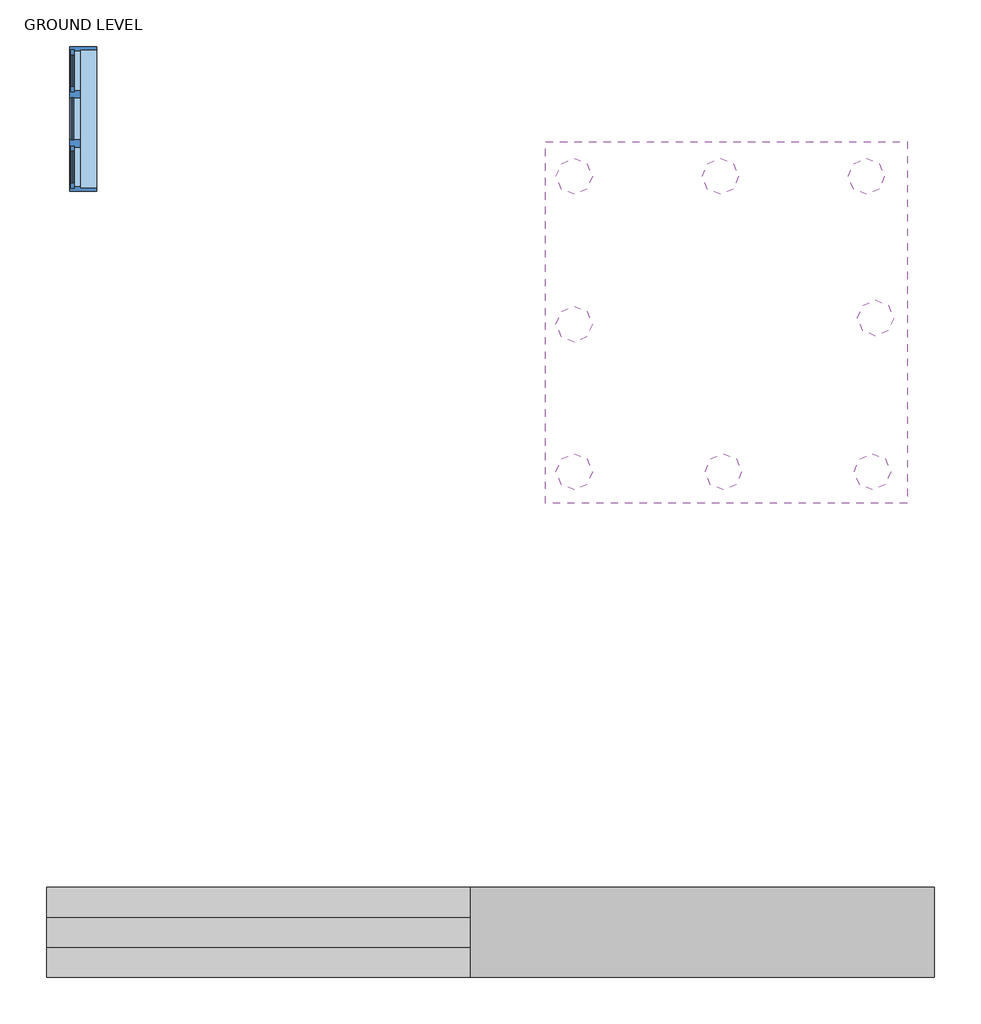
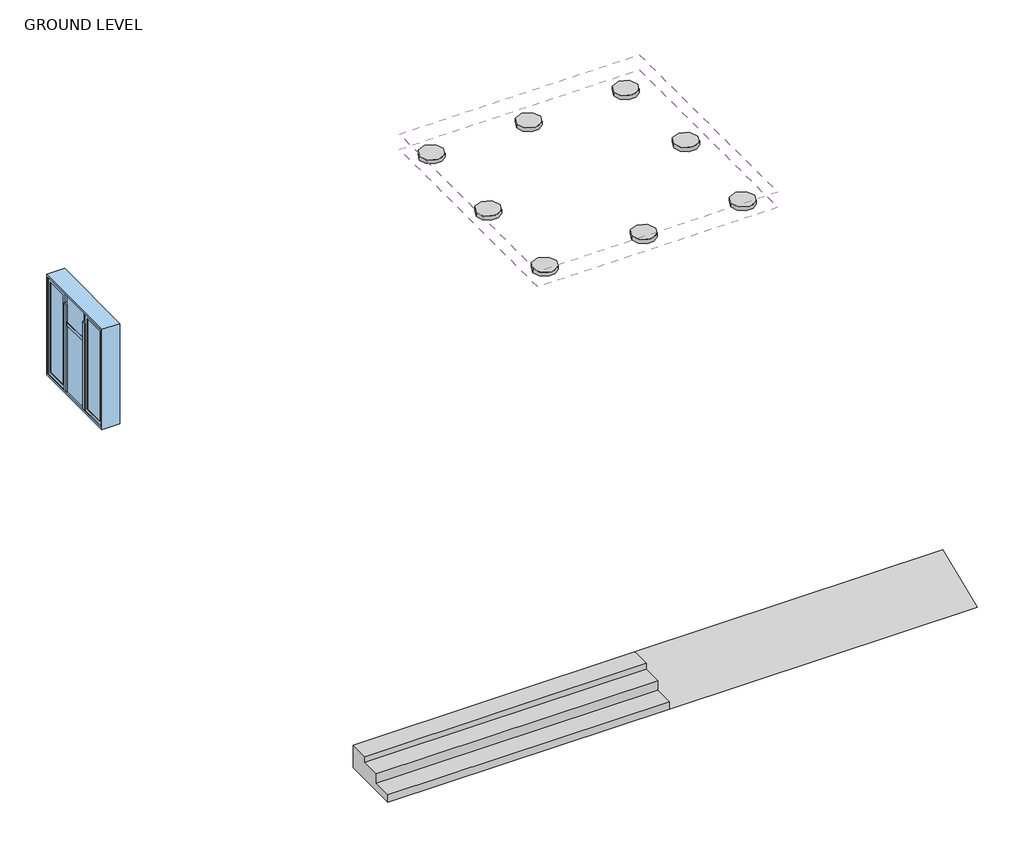
# One storey, incomplete: 8 light fixtures, 2 coverings, 2 proxies, 1 window.
"""IFC4 building model written with IfcOpenShell, lengths in millimetres."""

from ifc_helpers import new_model, si_unit, frame, origin, place, context, project, spatial, polyline, outline, extrude, transform, mapped, element, save
from components import generic_models_21_generic_models_21_217a5a39, generic_models_22_generic_models_22_fd5cddf6, family1_family1_bfb63c4d, window_casement_triple_middle_transom_windows_4_x4_273a115f

model = new_model("IFC4")

# Units and contexts
model_context = context("Model", 3, world=origin())
ifc_project = project(units=[si_unit("LENGTHUNIT", "METRE", prefix="MILLI")], contexts=[model_context])

# Site, building, storey
site = spatial("IfcSite", under=ifc_project)
building = spatial("IfcBuilding", under=site)
storey = spatial("IfcBuildingStorey", under=building, Name="GROUND LEVEL", Elevation=0.0)

# Proxies
placement = place(None, origin())
generic_models_21_generic_models_21_shape = generic_models_21_generic_models_21_217a5a39(model_context)
element("IfcBuildingElementProxy", 1, Name="Generic Models 21 : Generic Models 21", ObjectType="Generic Models 21 : Generic Models 21", at=placement, inside=storey, context=model_context, shape_type="MappedRepresentation", body=[
    mapped(generic_models_21_generic_models_21_shape, transform((0.0, 0.0, 0.0), x_axis=(1.0, 0.0, 0.0), y_axis=(0.0, 1.0, 0.0), z_axis=(0.0, 0.0, 1.0))),
])
generic_models_22_generic_models_22_shape = generic_models_22_generic_models_22_fd5cddf6(model_context)
element("IfcBuildingElementProxy", 2, Name="Generic Models 22 : Generic Models 22", ObjectType="Generic Models 22 : Generic Models 22", at=placement, inside=storey, context=model_context, shape_type="MappedRepresentation", body=[
    mapped(generic_models_22_generic_models_22_shape, transform((0.0, 0.0, 0.0), x_axis=(1.0, 0.0, 0.0), y_axis=(0.0, 1.0, 0.0), z_axis=(0.0, 0.0, 1.0))),
])

# Coverings
element("IfcCovering", 3, ObjectType="WHITE CEILING 2\"", at=placement, inside=storey, context=model_context, shape_type="SweptSolid", body=[
    extrude(outline(polyline([(-2635.3607439, -3293.8842658), (-2635.3607439, -6341.8842658), (-5683.3607439, -6341.8842658), (-5683.3607439, -3293.8842658), (-2635.3607439, -3293.8842658)])), frame((0.0, 0.0, 3225.8), z_axis=(0.0, 0.0, 1.0), x_axis=(1.0, 0.0, 0.0)), (0.0, 0.0, 1.0), 107.95),
])
element("IfcCovering", 4, ObjectType="WHITE CEILING 2\"", at=placement, inside=storey, context=model_context, shape_type="SweptSolid", body=[
    extrude(outline(polyline([(-2635.3607439, -3293.8842658), (-2635.3607439, -6341.8842658), (-5683.3607439, -6341.8842658), (-5683.3607439, -3293.8842658), (-2635.3607439, -3293.8842658)]), holes=[polyline([(-3067.1607439, -3725.6842658), (-5251.5607439, -3725.6842658), (-5251.5607439, -5910.0842658), (-3067.1607439, -5910.0842658), (-3067.1607439, -3725.6842658)])]), frame((0.0, 0.0, 3022.6), z_axis=(0.0, 0.0, 1.0), x_axis=(1.0, 0.0, 0.0)), (0.0, 0.0, 1.0), 107.95),
    extrude(outline(polyline([(-3371.9607439, -4030.4842658), (-3371.9607439, -5605.2842658), (-4946.7607439, -5605.2842658), (-4946.7607439, -4030.4842658), (-3371.9607439, -4030.4842658)])), frame((0.0, 0.0, 3022.6), z_axis=(0.0, 0.0, 1.0), x_axis=(1.0, 0.0, 0.0)), (0.0, 0.0, 1.0), 107.95),
])

# Light fixtures
family1_family1_shape = family1_family1_bfb63c4d(model_context)
element("IfcLightFixture", 5, ObjectType="Family1 : Family1", at=placement, inside=storey, context=model_context, shape_type="MappedRepresentation", body=[
    mapped(family1_family1_shape, transform((-5442.0607439, -3585.9842658, 584.2), x_axis=(1.0, 0.0, 0.0), y_axis=(0.0, 1.0, 0.0), z_axis=(0.0, 0.0, 1.0))),
])
element("IfcLightFixture", 6, ObjectType="Family1 : Family1", at=placement, inside=storey, context=model_context, shape_type="MappedRepresentation", body=[
    mapped(family1_family1_shape, transform((-2978.2607439, -3585.9842658, 584.2), x_axis=(1.0, 0.0, 0.0), y_axis=(0.0, 1.0, 0.0), z_axis=(0.0, 0.0, 1.0))),
])
element("IfcLightFixture", 7, ObjectType="Family1 : Family1", at=placement, inside=storey, context=model_context, shape_type="MappedRepresentation", body=[
    mapped(family1_family1_shape, transform((-4210.1607439, -3585.9842658, 584.2), x_axis=(1.0, 0.0, 0.0), y_axis=(0.0, 1.0, 0.0), z_axis=(0.0, 0.0, 1.0))),
])
element("IfcLightFixture", 8, ObjectType="Family1 : Family1", at=placement, inside=storey, context=model_context, shape_type="MappedRepresentation", body=[
    mapped(family1_family1_shape, transform((-5442.0607439, -6075.1842658, 584.2), x_axis=(1.0, 0.0, 0.0), y_axis=(0.0, 1.0, 0.0), z_axis=(0.0, 0.0, 1.0))),
])
element("IfcLightFixture", 9, ObjectType="Family1 : Family1", at=placement, inside=storey, context=model_context, shape_type="MappedRepresentation", body=[
    mapped(family1_family1_shape, transform((-5442.0607439, -4830.5842658, 584.2), x_axis=(1.0, 0.0, 0.0), y_axis=(0.0, 1.0, 0.0), z_axis=(0.0, 0.0, 1.0))),
])
element("IfcLightFixture", 10, ObjectType="Family1 : Family1", at=placement, inside=storey, context=model_context, shape_type="MappedRepresentation", body=[
    mapped(family1_family1_shape, transform((-2927.4607439, -6075.1842658, 584.2), x_axis=(1.0, 0.0, 0.0), y_axis=(0.0, 1.0, 0.0), z_axis=(0.0, 0.0, 1.0))),
])
element("IfcLightFixture", 11, ObjectType="Family1 : Family1", at=placement, inside=storey, context=model_context, shape_type="MappedRepresentation", body=[
    mapped(family1_family1_shape, transform((-4184.7607439, -6075.1842658, 584.2), x_axis=(1.0, 0.0, 0.0), y_axis=(0.0, 1.0, 0.0), z_axis=(0.0, 0.0, 1.0))),
])
element("IfcLightFixture", 12, ObjectType="Family1 : Family1", at=placement, inside=storey, context=model_context, shape_type="MappedRepresentation", body=[
    mapped(family1_family1_shape, transform((-2902.0607439, -4779.7842658, 584.2), x_axis=(1.0, 0.0, 0.0), y_axis=(0.0, 1.0, 0.0), z_axis=(0.0, 0.0, 1.0))),
])

# Window
window_casement_triple_middle_transom_windows_4_x4_shape = window_casement_triple_middle_transom_windows_4_x4_273a115f(model_context)
element("IfcWindow", 13, ObjectType="Window-Casement-Triple-Middle-Transom : WINDOWS 4'X4'", at=placement, inside=storey, context=model_context, shape_type="MappedRepresentation", body=[
    mapped(window_casement_triple_middle_transom_windows_4_x4_shape, transform((-9583.8482439, -3100.8442658, 0.0), x_axis=(0.0, 1.0, 0.0), y_axis=(-1.0, 0.0, 0.0), z_axis=(0.0, 0.0, 1.0))),
])

save(model, "model.ifc")

# Revit data of these elements
# Type "WHITE CEILING 2\""
#   Assembly Code = "C3030220"
#   built-in parameter 1002203 = 1 (stored number, unit not read)
#   built-in parameter 1002202 = 1 (stored number, unit not read)
#   Layers, outside or top first: 0' - 3 5/8" "Metal Stud Layer" (function 1); 0' - 0 5/8" "Clad - White" (function 5)
# Type "Family1 : Family1"
#   Photometric Web File = "generic"
#   Wattage = 12.1178 W
#   built-in parameter 1150110 = 1 (stored number, unit not read)
#   built-in parameter 1114217 = 1 (stored number, unit not read)
#   Tilt Angle = 60.00°
#   built-in parameter 1150109 = 1 (stored number, unit not read)
#   built-in parameter 1150113 = 1 (stored number, unit not read)
#   Lumens = 1800 lm
#   built-in parameter 1150115 = 1 (stored number, unit not read)
#   built-in parameter 1150105 = 143.239 (stored number, unit not read)
#   built-in parameter 1150112 = 1 (stored number, unit not read)
#   built-in parameter 1150114 = 1 (stored number, unit not read)
#   built-in parameter 1150107 = 3000 (stored number, unit not read)
#   built-in parameter 1150106 = 1.43239 (stored number, unit not read)
#   Emit from Circle Diameter = 2' - 0"
#   built-in parameter 1150104 = 13.8 (stored number, unit not read)
#   built-in parameter 1114218 = 1 (stored number, unit not read)
#   built-in parameter 1150133 = 10 (stored number, unit not read)
#   built-in parameter 1150132 = 2
#   Color Filter = 16777215
#   Emit Shape Visible in Rendering = no
#   Dimming Lamp Color Temperature Shift = (empty or 0)
#   Default Elevation = 0
# Type "Window-Casement-Triple-Middle-Transom : WINDOWS 4'X4'"
#   Type Mark = "21"
#   Fire Rating = "0.5h"
#   Assembly Code = "B2020100"
#   Analytic Construction = "Double glazing - domestic"
#   Window Width = 1' - 4"
#   Window Inset [instance default] = 0' - 0 5/8"
#   Wall Thickness [instance default] = 0' - 6"
#   Visual Light Transmittance = 0.81
#   Transom Height Ratio = 0.3
#   Thermal Resistance (R) = 1.8146 (h·ft²·°F)/BTU
#   Solar Heat Gain Coefficient = 0.76
#   Rough Width = 4' - 0 1/2"
#   Rough Height = 4' - 5 1/2"
#   Heat Transfer Coefficient (U) = 0.5511 BTU/(h·ft²·°F)
#   Height = 4' - 5"
#   Transom Height = 1' - 3.9"
#   Frame Gap 3 [instance default] = 0' - 1 83/128"
#   Frame Gap 2 [instance default] = 0' - 0 5/8"
#   Frame Gap 1 = 0' - 1 51/128"
#   Default Sill Height = 3' - 0"
#   Width = 4' - 0"
#   Frame Material = Metal - Aluminum
#   Glass Panel Material = Glass
#   Wall Closure = (empty or 0)
# Element 1 (IfcBuildingElementProxy, "Generic Models 21 : Generic Models 21")
#   Phase Created = New Construction
#   Materials on its faces: "CAST IN PLACE STAIRS"
# Element 2 (IfcBuildingElementProxy, "Generic Models 22 : Generic Models 22")
#   Phase Created = New Construction
#   Materials on its faces: "CAST IN PLACE STAIRS"
# Element 3 (IfcCovering, "WHITE CEILING 2\"")
#   Height Offset From Level = 10' - 7"
#   Phase Created = New Construction
#   Materials on its faces: "Clad - White", "Metal Stud Layer"
# Element 4 (IfcCovering, "WHITE CEILING 2\"")
#   Height Offset From Level = 9' - 11"
#   Phase Created = New Construction
#   Materials on its faces: "Clad - White", "Metal Stud Layer"
# Element 5 (IfcLightFixture, "Family1 : Family1")
#   Mark = "1"
#   Phase Created = New Construction
# Element 6 (IfcLightFixture, "Family1 : Family1")
#   Mark = "2"
#   Phase Created = New Construction
# Element 7 (IfcLightFixture, "Family1 : Family1")
#   Mark = "3"
#   Phase Created = New Construction
# Element 8 (IfcLightFixture, "Family1 : Family1")
#   Mark = "4"
#   Phase Created = New Construction
# Element 9 (IfcLightFixture, "Family1 : Family1")
#   Mark = "5"
#   Phase Created = New Construction
# Element 10 (IfcLightFixture, "Family1 : Family1")
#   Mark = "6"
#   Phase Created = New Construction
# Element 11 (IfcLightFixture, "Family1 : Family1")
#   Mark = "7"
#   Phase Created = New Construction
# Element 12 (IfcLightFixture, "Family1 : Family1")
#   Mark = "8"
#   Phase Created = New Construction
# Element 13 (IfcWindow, "Window-Casement-Triple-Middle-Transom : WINDOWS 4'X4'")
#   Mark = "21"
#   Window Inset = 0' - 0 5/8"
#   Frame Gap 3 = 0' - 1 83/128"
#   Frame Gap 2 = 0' - 0 5/8"
#   Phase Created = New Construction
#   Materials on its faces: "Metal - Aluminum", "Glass"
# Materials
#   "Metal Stud Layer": class "Metal", colour RGB 199 199 199, transparency 0, Description = "Light gauge steel framing, thermal air layer", Cost = 0
#   "Clad - White": class "Wood", colour RGB 242 242 238, transparency 0, Cost = 0
#   "Metal - Aluminum": class "Metal", colour RGB 247 247 247, transparency 0, Cost = 0
#   "Glass": class "Glass", colour RGB 0 128 192, transparency 0.75, Description = "Soda Lime Glass", Cost = 0
#   "CAST IN PLACE STAIRS": class "Generic", colour RGB 120 120 120, transparency 0, Cost = 0
